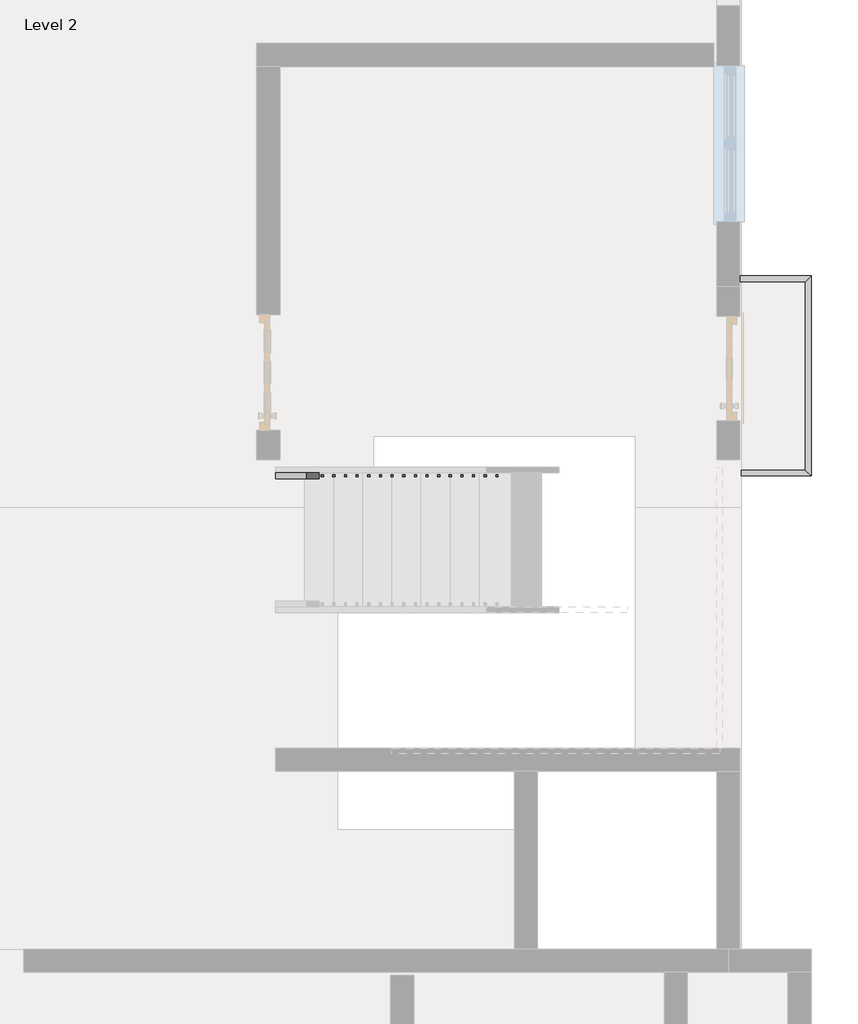
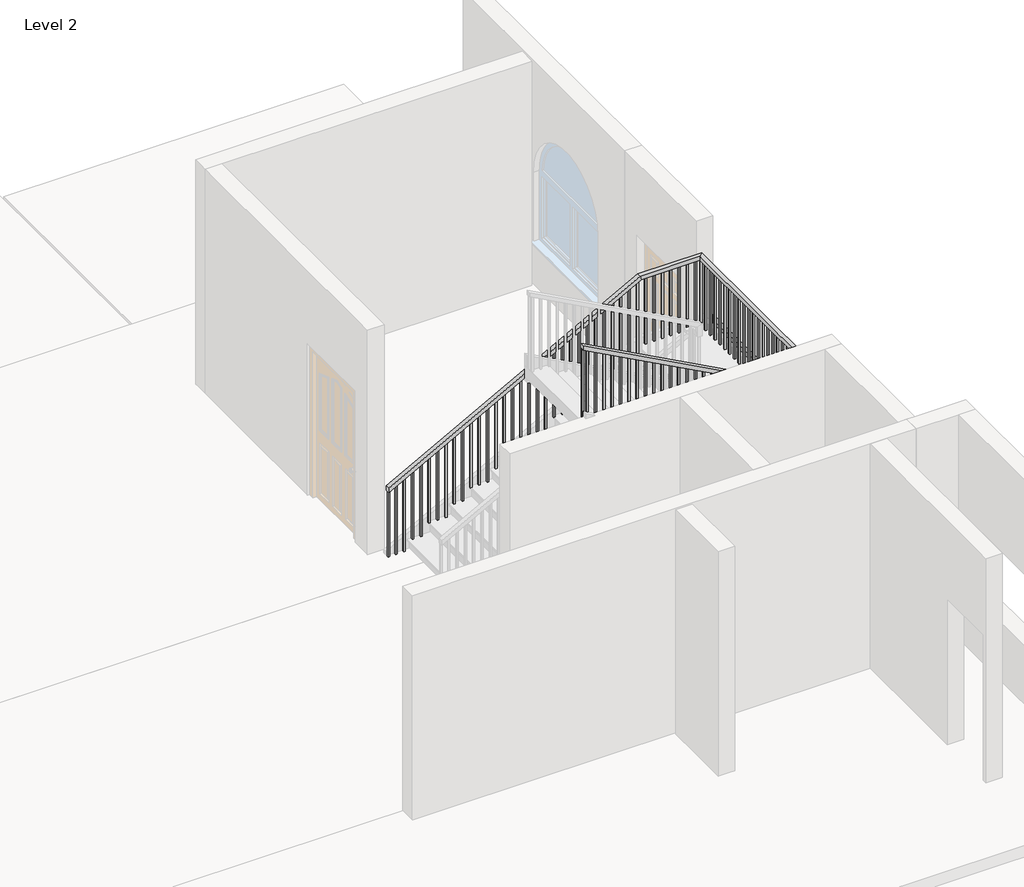
# One storey, part 6 of 7: 2 railings.
"""IFC4 building model written with IfcOpenShell, lengths in millimetres."""

from ifc_helpers import new_model, si_unit, frame, origin, place, context, project, spatial, polyline, outline, extrude, faceted_brep, element, save

model = new_model("IFC4")

# Units and contexts
model_context = context("Model", 3, world=origin())
ifc_project = project(units=[si_unit("LENGTHUNIT", "METRE", prefix="MILLI")], contexts=[model_context])

# Site, building, storey
site = spatial("IfcSite", under=ifc_project)
building = spatial("IfcBuilding", under=site)
storey = spatial("IfcBuildingStorey", under=building, Name="Level 2", Elevation=3048.0)

# Railings
placement = place(None, origin())
element("IfcRailing", 1, ObjectType="Handrail - Rectangular", at=placement, inside=storey, context=model_context, shape_type="SolidModel", body=[
    faceted_brep([(5863.1890963, 3183.81308, 3962.4), (5863.1890963, 3183.81308, 3911.6), (5863.1890963, 3133.01308, 3911.6), (5863.1890963, 3133.01308, 3962.4), (6485.4890963, 3183.81308, 3962.4), (6485.4890963, 3183.81308, 3911.6), (6434.6890963, 3133.01308, 3911.6), (6434.6890963, 3133.01308, 3962.4), (6485.4890963, 1439.3962251, 3962.4), (6485.4890963, 1439.3962251, 3911.6), (6434.6890963, 1490.1962251, 3911.6), (6434.6890963, 1490.1962251, 3962.4), (5875.8890963, 1439.3962251, 3962.4), (5875.8890963, 1490.1962251, 3962.4), (5875.8890963, 1490.1962251, 3911.6), (5875.8890963, 1439.3962251, 3911.6)], [[[0, 1, 2, 3]], [[1, 0, 4, 5]], [[2, 1, 5, 6]], [[3, 2, 6, 7]], [[0, 3, 7, 4]], [[5, 4, 8, 9]], [[6, 5, 9, 10]], [[7, 6, 10, 11]], [[4, 7, 11, 8]], [[12, 13, 14, 15]], [[9, 8, 12, 15]], [[10, 9, 15, 14]], [[11, 10, 14, 13]], [[8, 11, 13, 12]]]),
    extrude(outline(polyline([(5961.6140963, 1474.3212251), (5961.6140963, 1455.2712251), (5942.5640963, 1455.2712251), (5942.5640963, 1474.3212251), (5961.6140963, 1474.3212251)])), frame((0.0, 0.0, 3048.0), z_axis=(0.0, 0.0, 1.0), x_axis=(1.0, 0.0, 0.0)), (0.0, 0.0, 1.0), 863.6),
    extrude(outline(polyline([(6063.2140963, 1474.3212251), (6063.2140963, 1455.2712251), (6044.1640963, 1455.2712251), (6044.1640963, 1474.3212251), (6063.2140963, 1474.3212251)])), frame((0.0, 0.0, 3048.0), z_axis=(0.0, 0.0, 1.0), x_axis=(1.0, 0.0, 0.0)), (0.0, 0.0, 1.0), 863.6),
    extrude(outline(polyline([(6164.8140963, 1474.3212251), (6164.8140963, 1455.2712251), (6145.7640963, 1455.2712251), (6145.7640963, 1474.3212251), (6164.8140963, 1474.3212251)])), frame((0.0, 0.0, 3048.0), z_axis=(0.0, 0.0, 1.0), x_axis=(1.0, 0.0, 0.0)), (0.0, 0.0, 1.0), 863.6),
    extrude(outline(polyline([(6266.4140963, 1474.3212251), (6266.4140963, 1455.2712251), (6247.3640963, 1455.2712251), (6247.3640963, 1474.3212251), (6266.4140963, 1474.3212251)])), frame((0.0, 0.0, 3048.0), z_axis=(0.0, 0.0, 1.0), x_axis=(1.0, 0.0, 0.0)), (0.0, 0.0, 1.0), 863.6),
    extrude(outline(polyline([(6368.0140963, 1474.3212251), (6368.0140963, 1455.2712251), (6348.9640963, 1455.2712251), (6348.9640963, 1474.3212251), (6368.0140963, 1474.3212251)])), frame((0.0, 0.0, 3048.0), z_axis=(0.0, 0.0, 1.0), x_axis=(1.0, 0.0, 0.0)), (0.0, 0.0, 1.0), 863.6),
    extrude(outline(polyline([(6450.5640963, 1542.33808), (6469.6140963, 1542.33808), (6469.6140963, 1523.28808), (6450.5640963, 1523.28808), (6450.5640963, 1542.33808)])), frame((0.0, 0.0, 3048.0), z_axis=(0.0, 0.0, 1.0), x_axis=(1.0, 0.0, 0.0)), (0.0, 0.0, 1.0), 863.6),
    extrude(outline(polyline([(6450.5640963, 1643.93808), (6469.6140963, 1643.93808), (6469.6140963, 1624.88808), (6450.5640963, 1624.88808), (6450.5640963, 1643.93808)])), frame((0.0, 0.0, 3048.0), z_axis=(0.0, 0.0, 1.0), x_axis=(1.0, 0.0, 0.0)), (0.0, 0.0, 1.0), 863.6),
    extrude(outline(polyline([(6450.5640963, 1745.53808), (6469.6140963, 1745.53808), (6469.6140963, 1726.48808), (6450.5640963, 1726.48808), (6450.5640963, 1745.53808)])), frame((0.0, 0.0, 3048.0), z_axis=(0.0, 0.0, 1.0), x_axis=(1.0, 0.0, 0.0)), (0.0, 0.0, 1.0), 863.6),
    extrude(outline(polyline([(6450.5640963, 1847.13808), (6469.6140963, 1847.13808), (6469.6140963, 1828.08808), (6450.5640963, 1828.08808), (6450.5640963, 1847.13808)])), frame((0.0, 0.0, 3048.0), z_axis=(0.0, 0.0, 1.0), x_axis=(1.0, 0.0, 0.0)), (0.0, 0.0, 1.0), 863.6),
    extrude(outline(polyline([(6450.5640963, 1948.73808), (6469.6140963, 1948.73808), (6469.6140963, 1929.68808), (6450.5640963, 1929.68808), (6450.5640963, 1948.73808)])), frame((0.0, 0.0, 3048.0), z_axis=(0.0, 0.0, 1.0), x_axis=(1.0, 0.0, 0.0)), (0.0, 0.0, 1.0), 863.6),
    extrude(outline(polyline([(6450.5640963, 2050.33808), (6469.6140963, 2050.33808), (6469.6140963, 2031.28808), (6450.5640963, 2031.28808), (6450.5640963, 2050.33808)])), frame((0.0, 0.0, 3048.0), z_axis=(0.0, 0.0, 1.0), x_axis=(1.0, 0.0, 0.0)), (0.0, 0.0, 1.0), 863.6),
    extrude(outline(polyline([(6450.5640963, 2151.93808), (6469.6140963, 2151.93808), (6469.6140963, 2132.88808), (6450.5640963, 2132.88808), (6450.5640963, 2151.93808)])), frame((0.0, 0.0, 3048.0), z_axis=(0.0, 0.0, 1.0), x_axis=(1.0, 0.0, 0.0)), (0.0, 0.0, 1.0), 863.6),
    extrude(outline(polyline([(6450.5640963, 2253.53808), (6469.6140963, 2253.53808), (6469.6140963, 2234.48808), (6450.5640963, 2234.48808), (6450.5640963, 2253.53808)])), frame((0.0, 0.0, 3048.0), z_axis=(0.0, 0.0, 1.0), x_axis=(1.0, 0.0, 0.0)), (0.0, 0.0, 1.0), 863.6),
    extrude(outline(polyline([(6450.5640963, 2355.13808), (6469.6140963, 2355.13808), (6469.6140963, 2336.08808), (6450.5640963, 2336.08808), (6450.5640963, 2355.13808)])), frame((0.0, 0.0, 3048.0), z_axis=(0.0, 0.0, 1.0), x_axis=(1.0, 0.0, 0.0)), (0.0, 0.0, 1.0), 863.6),
    extrude(outline(polyline([(6450.5640963, 2456.73808), (6469.6140963, 2456.73808), (6469.6140963, 2437.68808), (6450.5640963, 2437.68808), (6450.5640963, 2456.73808)])), frame((0.0, 0.0, 3048.0), z_axis=(0.0, 0.0, 1.0), x_axis=(1.0, 0.0, 0.0)), (0.0, 0.0, 1.0), 863.6),
    extrude(outline(polyline([(6450.5640963, 2558.33808), (6469.6140963, 2558.33808), (6469.6140963, 2539.28808), (6450.5640963, 2539.28808), (6450.5640963, 2558.33808)])), frame((0.0, 0.0, 3048.0), z_axis=(0.0, 0.0, 1.0), x_axis=(1.0, 0.0, 0.0)), (0.0, 0.0, 1.0), 863.6),
    extrude(outline(polyline([(6450.5640963, 2659.93808), (6469.6140963, 2659.93808), (6469.6140963, 2640.88808), (6450.5640963, 2640.88808), (6450.5640963, 2659.93808)])), frame((0.0, 0.0, 3048.0), z_axis=(0.0, 0.0, 1.0), x_axis=(1.0, 0.0, 0.0)), (0.0, 0.0, 1.0), 863.6),
    extrude(outline(polyline([(6450.5640963, 2761.53808), (6469.6140963, 2761.53808), (6469.6140963, 2742.48808), (6450.5640963, 2742.48808), (6450.5640963, 2761.53808)])), frame((0.0, 0.0, 3048.0), z_axis=(0.0, 0.0, 1.0), x_axis=(1.0, 0.0, 0.0)), (0.0, 0.0, 1.0), 863.6),
    extrude(outline(polyline([(6450.5640963, 2863.13808), (6469.6140963, 2863.13808), (6469.6140963, 2844.08808), (6450.5640963, 2844.08808), (6450.5640963, 2863.13808)])), frame((0.0, 0.0, 3048.0), z_axis=(0.0, 0.0, 1.0), x_axis=(1.0, 0.0, 0.0)), (0.0, 0.0, 1.0), 863.6),
    extrude(outline(polyline([(6450.5640963, 2964.73808), (6469.6140963, 2964.73808), (6469.6140963, 2945.68808), (6450.5640963, 2945.68808), (6450.5640963, 2964.73808)])), frame((0.0, 0.0, 3048.0), z_axis=(0.0, 0.0, 1.0), x_axis=(1.0, 0.0, 0.0)), (0.0, 0.0, 1.0), 863.6),
    extrude(outline(polyline([(6450.5640963, 3066.33808), (6469.6140963, 3066.33808), (6469.6140963, 3047.28808), (6450.5640963, 3047.28808), (6450.5640963, 3066.33808)])), frame((0.0, 0.0, 3048.0), z_axis=(0.0, 0.0, 1.0), x_axis=(1.0, 0.0, 0.0)), (0.0, 0.0, 1.0), 863.6),
    extrude(outline(polyline([(6361.6640963, 3148.88808), (6361.6640963, 3167.93808), (6380.7140963, 3167.93808), (6380.7140963, 3148.88808), (6361.6640963, 3148.88808)])), frame((0.0, 0.0, 3048.0), z_axis=(0.0, 0.0, 1.0), x_axis=(1.0, 0.0, 0.0)), (0.0, 0.0, 1.0), 863.6),
    extrude(outline(polyline([(6260.0640963, 3148.88808), (6260.0640963, 3167.93808), (6279.1140963, 3167.93808), (6279.1140963, 3148.88808), (6260.0640963, 3148.88808)])), frame((0.0, 0.0, 3048.0), z_axis=(0.0, 0.0, 1.0), x_axis=(1.0, 0.0, 0.0)), (0.0, 0.0, 1.0), 863.6),
    extrude(outline(polyline([(6158.4640963, 3148.88808), (6158.4640963, 3167.93808), (6177.5140963, 3167.93808), (6177.5140963, 3148.88808), (6158.4640963, 3148.88808)])), frame((0.0, 0.0, 3048.0), z_axis=(0.0, 0.0, 1.0), x_axis=(1.0, 0.0, 0.0)), (0.0, 0.0, 1.0), 863.6),
    extrude(outline(polyline([(6056.8640963, 3148.88808), (6056.8640963, 3167.93808), (6075.9140963, 3167.93808), (6075.9140963, 3148.88808), (6056.8640963, 3148.88808)])), frame((0.0, 0.0, 3048.0), z_axis=(0.0, 0.0, 1.0), x_axis=(1.0, 0.0, 0.0)), (0.0, 0.0, 1.0), 863.6),
    extrude(outline(polyline([(5955.2640963, 3148.88808), (5955.2640963, 3167.93808), (5974.3140963, 3167.93808), (5974.3140963, 3148.88808), (5955.2640963, 3148.88808)])), frame((0.0, 0.0, 3048.0), z_axis=(0.0, 0.0, 1.0), x_axis=(1.0, 0.0, 0.0)), (0.0, 0.0, 1.0), 863.6),
    extrude(outline(polyline([(6450.5640963, 1474.3212251), (6469.6140963, 1474.3212251), (6469.6140963, 1455.2712251), (6450.5640963, 1455.2712251), (6450.5640963, 1474.3212251)])), frame((0.0, 0.0, 3048.0), z_axis=(0.0, 0.0, 1.0), x_axis=(1.0, 0.0, 0.0)), (0.0, 0.0, 1.0), 863.6),
    extrude(outline(polyline([(6450.5640963, 3148.88808), (6450.5640963, 3167.93808), (6469.6140963, 3167.93808), (6469.6140963, 3148.88808), (6450.5640963, 3148.88808)])), frame((0.0, 0.0, 3048.0), z_axis=(0.0, 0.0, 1.0), x_axis=(1.0, 0.0, 0.0)), (0.0, 0.0, 1.0), 863.6),
    extrude(outline(polyline([(5894.9390963, 1474.3212251), (5894.9390963, 1455.2712251), (5875.8890963, 1455.2712251), (5875.8890963, 1474.3212251), (5894.9390963, 1474.3212251)])), frame((0.0, 0.0, 3048.0), z_axis=(0.0, 0.0, 1.0), x_axis=(1.0, 0.0, 0.0)), (0.0, 0.0, 1.0), 863.6),
    extrude(outline(polyline([(5863.1890963, 3148.88808), (5863.1890963, 3167.93808), (5882.2390963, 3167.93808), (5882.2390963, 3148.88808), (5863.1890963, 3148.88808)])), frame((0.0, 0.0, 3048.0), z_axis=(0.0, 0.0, 1.0), x_axis=(1.0, 0.0, 0.0)), (0.0, 0.0, 1.0), 863.6),
])
element("IfcRailing", 2, ObjectType="Handrail - Rectangular", at=placement, inside=storey, context=model_context, shape_type="SolidModel", body=[
    faceted_brep([(1811.8890963, 1464.7962251, 4100.9454545), (1811.8890963, 1464.7962251, 4043.1709673), (1811.8890963, 1413.9962251, 4043.1709673), (1811.8890963, 1413.9962251, 4100.9454545), (4881.0326586, 1464.7962251, 5763.4909091), (4893.9079172, 1464.7962251, 5712.6909091), (4893.9079172, 1413.9962251, 5712.6909091), (4881.0326586, 1413.9962251, 5763.4909091), (5659.9890963, 1464.7962251, 5763.4909091), (5659.9890963, 1464.7962251, 5712.6909091), (5609.1890963, 1413.9962251, 5712.6909091), (5609.1890963, 1413.9962251, 5763.4909091), (5659.9890963, -935.5037749, 5763.4909091), (5659.9890963, -935.5037749, 5712.6909091), (5609.1890963, -884.7037749, 5712.6909091), (5609.1890963, -884.7037749, 5763.4909091), (5137.6756039, -935.5037749, 5763.4909091), (5124.8392301, -935.5037749, 5712.6909091), (5124.8392301, -884.7037749, 5712.6909091), (5137.6756039, -884.7037749, 5763.4909091), (2827.8890963, -935.5037749, 7010.4), (2827.8890963, -884.7037749, 7010.4), (2827.8890963, -884.7037749, 6952.6704456), (2827.8890963, -935.5037749, 6952.6704456)], [[[0, 1, 2, 3]], [[1, 0, 4, 5]], [[2, 1, 5, 6]], [[3, 2, 6, 7]], [[0, 3, 7, 4]], [[5, 4, 8, 9]], [[6, 5, 9, 10]], [[7, 6, 10, 11]], [[4, 7, 11, 8]], [[9, 8, 12, 13]], [[10, 9, 13, 14]], [[11, 10, 14, 15]], [[8, 11, 15, 12]], [[13, 12, 16, 17]], [[14, 13, 17, 18]], [[15, 14, 18, 19]], [[12, 15, 19, 16]], [[20, 21, 22, 23]], [[17, 16, 20, 23]], [[18, 17, 23, 22]], [[19, 18, 22, 21]], [[16, 19, 21, 20]]]),
    extrude(outline(polyline([(6923.5858236, 2881.8640963), (5957.4545455, 2881.8640963), (5957.4545455, 2900.9140963), (6913.2664983, 2900.9140963), (6923.5858236, 2881.8640963)])), frame((0.0, -919.6287749, 0.0), z_axis=(0.0, 1.0, 0.0), x_axis=(0.0, 0.0, 1.0)), (0.0, 0.0, 1.0), 19.05),
    extrude(outline(polyline([(6868.5494219, 2983.4640963), (5957.4545455, 2983.4640963), (5957.4545455, 3002.5140963), (6858.2300965, 3002.5140963), (6868.5494219, 2983.4640963)])), frame((0.0, -919.6287749, 0.0), z_axis=(0.0, 1.0, 0.0), x_axis=(0.0, 0.0, 1.0)), (0.0, 0.0, 1.0), 19.05),
    extrude(outline(polyline([(6813.8377681, 3085.0640963), (5818.9090909, 3085.0640963), (5818.9090909, 3104.1140963), (6803.553866, 3104.1140963), (6813.8377681, 3085.0640963)])), frame((0.0, -919.6287749, 0.0), z_axis=(0.0, 1.0, 0.0), x_axis=(0.0, 0.0, 1.0)), (0.0, 0.0, 1.0), 19.05),
    extrude(outline(polyline([(6758.9902905, 3186.6640963), (5818.9090909, 3186.6640963), (5818.9090909, 3205.7140963), (6748.7063885, 3205.7140963), (6758.9902905, 3186.6640963)])), frame((0.0, -919.6287749, 0.0), z_axis=(0.0, 1.0, 0.0), x_axis=(0.0, 0.0, 1.0)), (0.0, 0.0, 1.0), 19.05),
    extrude(outline(polyline([(6704.1428129, 3288.2640963), (5818.9090909, 3288.2640963), (5818.9090909, 3307.3140963), (6693.8589109, 3307.3140963), (6704.1428129, 3288.2640963)])), frame((0.0, -919.6287749, 0.0), z_axis=(0.0, 1.0, 0.0), x_axis=(0.0, 0.0, 1.0)), (0.0, 0.0, 1.0), 19.05),
    extrude(outline(polyline([(6649.2953354, 3389.8640963), (5680.3636364, 3389.8640963), (5680.3636364, 3408.9140963), (6639.0114333, 3408.9140963), (6649.2953354, 3389.8640963)])), frame((0.0, -919.6287749, 0.0), z_axis=(0.0, 1.0, 0.0), x_axis=(0.0, 0.0, 1.0)), (0.0, 0.0, 1.0), 19.05),
    extrude(outline(polyline([(6594.4478578, 3491.4640963), (5680.3636364, 3491.4640963), (5680.3636364, 3510.5140963), (6584.1639558, 3510.5140963), (6594.4478578, 3491.4640963)])), frame((0.0, -919.6287749, 0.0), z_axis=(0.0, 1.0, 0.0), x_axis=(0.0, 0.0, 1.0)), (0.0, 0.0, 1.0), 19.05),
    extrude(outline(polyline([(6539.6003803, 3593.0640963), (5541.8181818, 3593.0640963), (5541.8181818, 3612.1140963), (6529.3164782, 3612.1140963), (6539.6003803, 3593.0640963)])), frame((0.0, -919.6287749, 0.0), z_axis=(0.0, 1.0, 0.0), x_axis=(0.0, 0.0, 1.0)), (0.0, 0.0, 1.0), 19.05),
    extrude(outline(polyline([(6484.7529027, 3694.6640963), (5541.8181818, 3694.6640963), (5541.8181818, 3713.7140963), (6474.4690007, 3713.7140963), (6484.7529027, 3694.6640963)])), frame((0.0, -919.6287749, 0.0), z_axis=(0.0, 1.0, 0.0), x_axis=(0.0, 0.0, 1.0)), (0.0, 0.0, 1.0), 19.05),
    extrude(outline(polyline([(6429.9054252, 3796.2640963), (5541.8181818, 3796.2640963), (5541.8181818, 3815.3140963), (6419.6215231, 3815.3140963), (6429.9054252, 3796.2640963)])), frame((0.0, -919.6287749, 0.0), z_axis=(0.0, 1.0, 0.0), x_axis=(0.0, 0.0, 1.0)), (0.0, 0.0, 1.0), 19.05),
    extrude(outline(polyline([(6375.1307062, 3897.8640963), (5403.2727273, 3897.8640963), (5403.2727273, 3916.9140963), (6364.8113809, 3916.9140963), (6375.1307062, 3897.8640963)])), frame((0.0, -919.6287749, 0.0), z_axis=(0.0, 1.0, 0.0), x_axis=(0.0, 0.0, 1.0)), (0.0, 0.0, 1.0), 19.05),
    extrude(outline(polyline([(6320.0943044, 3999.4640963), (5403.2727273, 3999.4640963), (5403.2727273, 4018.5140963), (6309.7749791, 4018.5140963), (6320.0943044, 3999.4640963)])), frame((0.0, -919.6287749, 0.0), z_axis=(0.0, 1.0, 0.0), x_axis=(0.0, 0.0, 1.0)), (0.0, 0.0, 1.0), 19.05),
    extrude(outline(polyline([(6265.3629925, 4101.0640963), (5264.7272727, 4101.0640963), (5264.7272727, 4120.1140963), (6255.0790904, 4120.1140963), (6265.3629925, 4101.0640963)])), frame((0.0, -919.6287749, 0.0), z_axis=(0.0, 1.0, 0.0), x_axis=(0.0, 0.0, 1.0)), (0.0, 0.0, 1.0), 19.05),
    extrude(outline(polyline([(6210.5155149, 4202.6640963), (5264.7272727, 4202.6640963), (5264.7272727, 4221.7140963), (6200.2316129, 4221.7140963), (6210.5155149, 4202.6640963)])), frame((0.0, -919.6287749, 0.0), z_axis=(0.0, 1.0, 0.0), x_axis=(0.0, 0.0, 1.0)), (0.0, 0.0, 1.0), 19.05),
    extrude(outline(polyline([(6155.6680374, 4304.2640963), (5264.7272727, 4304.2640963), (5264.7272727, 4323.3140963), (6145.3841353, 4323.3140963), (6155.6680374, 4304.2640963)])), frame((0.0, -919.6287749, 0.0), z_axis=(0.0, 1.0, 0.0), x_axis=(0.0, 0.0, 1.0)), (0.0, 0.0, 1.0), 19.05),
    extrude(outline(polyline([(6100.8205598, 4405.8640963), (5126.1818182, 4405.8640963), (5126.1818182, 4424.9140963), (6090.5366578, 4424.9140963), (6100.8205598, 4405.8640963)])), frame((0.0, -919.6287749, 0.0), z_axis=(0.0, 1.0, 0.0), x_axis=(0.0, 0.0, 1.0)), (0.0, 0.0, 1.0), 19.05),
    extrude(outline(polyline([(6045.9730823, 4507.4640963), (5126.1818182, 4507.4640963), (5126.1818182, 4526.5140963), (6035.6891802, 4526.5140963), (6045.9730823, 4507.4640963)])), frame((0.0, -919.6287749, 0.0), z_axis=(0.0, 1.0, 0.0), x_axis=(0.0, 0.0, 1.0)), (0.0, 0.0, 1.0), 19.05),
    extrude(outline(polyline([(5991.1256047, 4609.0640963), (4987.6363636, 4609.0640963), (4987.6363636, 4628.1140963), (5980.8417027, 4628.1140963), (5991.1256047, 4609.0640963)])), frame((0.0, -919.6287749, 0.0), z_axis=(0.0, 1.0, 0.0), x_axis=(0.0, 0.0, 1.0)), (0.0, 0.0, 1.0), 19.05),
    extrude(outline(polyline([(5936.2781272, 4710.6640963), (4987.6363636, 4710.6640963), (4987.6363636, 4729.7140963), (5925.9942251, 4729.7140963), (5936.2781272, 4710.6640963)])), frame((0.0, -919.6287749, 0.0), z_axis=(0.0, 1.0, 0.0), x_axis=(0.0, 0.0, 1.0)), (0.0, 0.0, 1.0), 19.05),
    extrude(outline(polyline([(5881.4306496, 4812.2640963), (4987.6363636, 4812.2640963), (4987.6363636, 4831.3140963), (5871.1467476, 4831.3140963), (5881.4306496, 4812.2640963)])), frame((0.0, -919.6287749, 0.0), z_axis=(0.0, 1.0, 0.0), x_axis=(0.0, 0.0, 1.0)), (0.0, 0.0, 1.0), 19.05),
    extrude(outline(polyline([(5826.583172, 4913.8640963), (4849.0909091, 4913.8640963), (4849.0909091, 4932.9140963), (5816.29927, 4932.9140963), (5826.583172, 4913.8640963)])), frame((0.0, -919.6287749, 0.0), z_axis=(0.0, 1.0, 0.0), x_axis=(0.0, 0.0, 1.0)), (0.0, 0.0, 1.0), 19.05),
    extrude(outline(polyline([(5771.7356945, 5015.4640963), (4849.0909091, 5015.4640963), (4849.0909091, 5034.5140963), (5761.4517924, 5034.5140963), (5771.7356945, 5015.4640963)])), frame((0.0, -919.6287749, 0.0), z_axis=(0.0, 1.0, 0.0), x_axis=(0.0, 0.0, 1.0)), (0.0, 0.0, 1.0), 19.05),
    extrude(outline(polyline([(5716.8882169, 5117.0640963), (4849.0909091, 5117.0640963), (4849.0909091, 5136.1140963), (5706.6043149, 5136.1140963), (5716.8882169, 5117.0640963)])), frame((0.0, -919.6287749, 0.0), z_axis=(0.0, 1.0, 0.0), x_axis=(0.0, 0.0, 1.0)), (0.0, 0.0, 1.0), 19.05),
    extrude(outline(polyline([(5237.7140963, -919.6287749), (5218.6640963, -919.6287749), (5218.6640963, -900.5787749), (5237.7140963, -900.5787749), (5237.7140963, -919.6287749)])), frame((0.0, 0.0, 4849.0909091), z_axis=(0.0, 0.0, 1.0), x_axis=(1.0, 0.0, 0.0)), (0.0, 0.0, 1.0), 863.6),
    extrude(outline(polyline([(5339.3140963, -919.6287749), (5320.2640963, -919.6287749), (5320.2640963, -900.5787749), (5339.3140963, -900.5787749), (5339.3140963, -919.6287749)])), frame((0.0, 0.0, 4849.0909091), z_axis=(0.0, 0.0, 1.0), x_axis=(1.0, 0.0, 0.0)), (0.0, 0.0, 1.0), 863.6),
    extrude(outline(polyline([(5440.9140963, -919.6287749), (5421.8640963, -919.6287749), (5421.8640963, -900.5787749), (5440.9140963, -900.5787749), (5440.9140963, -919.6287749)])), frame((0.0, 0.0, 4849.0909091), z_axis=(0.0, 0.0, 1.0), x_axis=(1.0, 0.0, 0.0)), (0.0, 0.0, 1.0), 863.6),
    extrude(outline(polyline([(5542.5140963, -919.6287749), (5523.4640963, -919.6287749), (5523.4640963, -900.5787749), (5542.5140963, -900.5787749), (5542.5140963, -919.6287749)])), frame((0.0, 0.0, 4849.0909091), z_axis=(0.0, 0.0, 1.0), x_axis=(1.0, 0.0, 0.0)), (0.0, 0.0, 1.0), 863.6),
    extrude(outline(polyline([(5644.1140963, -887.8787749), (5644.1140963, -906.9287749), (5625.0640963, -906.9287749), (5625.0640963, -887.8787749), (5644.1140963, -887.8787749)])), frame((0.0, 0.0, 4849.0909091), z_axis=(0.0, 0.0, 1.0), x_axis=(1.0, 0.0, 0.0)), (0.0, 0.0, 1.0), 863.6),
    extrude(outline(polyline([(5644.1140963, -786.2787749), (5644.1140963, -805.3287749), (5625.0640963, -805.3287749), (5625.0640963, -786.2787749), (5644.1140963, -786.2787749)])), frame((0.0, 0.0, 4849.0909091), z_axis=(0.0, 0.0, 1.0), x_axis=(1.0, 0.0, 0.0)), (0.0, 0.0, 1.0), 863.6),
    extrude(outline(polyline([(5644.1140963, -684.6787749), (5644.1140963, -703.7287749), (5625.0640963, -703.7287749), (5625.0640963, -684.6787749), (5644.1140963, -684.6787749)])), frame((0.0, 0.0, 4849.0909091), z_axis=(0.0, 0.0, 1.0), x_axis=(1.0, 0.0, 0.0)), (0.0, 0.0, 1.0), 863.6),
    extrude(outline(polyline([(5644.1140963, -583.0787749), (5644.1140963, -602.1287749), (5625.0640963, -602.1287749), (5625.0640963, -583.0787749), (5644.1140963, -583.0787749)])), frame((0.0, 0.0, 4849.0909091), z_axis=(0.0, 0.0, 1.0), x_axis=(1.0, 0.0, 0.0)), (0.0, 0.0, 1.0), 863.6),
    extrude(outline(polyline([(5644.1140963, -481.4787749), (5644.1140963, -500.5287749), (5625.0640963, -500.5287749), (5625.0640963, -481.4787749), (5644.1140963, -481.4787749)])), frame((0.0, 0.0, 4849.0909091), z_axis=(0.0, 0.0, 1.0), x_axis=(1.0, 0.0, 0.0)), (0.0, 0.0, 1.0), 863.6),
    extrude(outline(polyline([(5644.1140963, -379.8787749), (5644.1140963, -398.9287749), (5625.0640963, -398.9287749), (5625.0640963, -379.8787749), (5644.1140963, -379.8787749)])), frame((0.0, 0.0, 4849.0909091), z_axis=(0.0, 0.0, 1.0), x_axis=(1.0, 0.0, 0.0)), (0.0, 0.0, 1.0), 863.6),
    extrude(outline(polyline([(5644.1140963, -278.2787749), (5644.1140963, -297.3287749), (5625.0640963, -297.3287749), (5625.0640963, -278.2787749), (5644.1140963, -278.2787749)])), frame((0.0, 0.0, 4849.0909091), z_axis=(0.0, 0.0, 1.0), x_axis=(1.0, 0.0, 0.0)), (0.0, 0.0, 1.0), 863.6),
    extrude(outline(polyline([(5644.1140963, -176.6787749), (5644.1140963, -195.7287749), (5625.0640963, -195.7287749), (5625.0640963, -176.6787749), (5644.1140963, -176.6787749)])), frame((0.0, 0.0, 4849.0909091), z_axis=(0.0, 0.0, 1.0), x_axis=(1.0, 0.0, 0.0)), (0.0, 0.0, 1.0), 863.6),
    extrude(outline(polyline([(5644.1140963, -75.0787749), (5644.1140963, -94.1287749), (5625.0640963, -94.1287749), (5625.0640963, -75.0787749), (5644.1140963, -75.0787749)])), frame((0.0, 0.0, 4849.0909091), z_axis=(0.0, 0.0, 1.0), x_axis=(1.0, 0.0, 0.0)), (0.0, 0.0, 1.0), 863.6),
    extrude(outline(polyline([(5644.1140963, 26.5212251), (5644.1140963, 7.4712251), (5625.0640963, 7.4712251), (5625.0640963, 26.5212251), (5644.1140963, 26.5212251)])), frame((0.0, 0.0, 4849.0909091), z_axis=(0.0, 0.0, 1.0), x_axis=(1.0, 0.0, 0.0)), (0.0, 0.0, 1.0), 863.6),
    extrude(outline(polyline([(5644.1140963, 128.1212251), (5644.1140963, 109.0712251), (5625.0640963, 109.0712251), (5625.0640963, 128.1212251), (5644.1140963, 128.1212251)])), frame((0.0, 0.0, 4849.0909091), z_axis=(0.0, 0.0, 1.0), x_axis=(1.0, 0.0, 0.0)), (0.0, 0.0, 1.0), 863.6),
    extrude(outline(polyline([(5644.1140963, 229.7212251), (5644.1140963, 210.6712251), (5625.0640963, 210.6712251), (5625.0640963, 229.7212251), (5644.1140963, 229.7212251)])), frame((0.0, 0.0, 4849.0909091), z_axis=(0.0, 0.0, 1.0), x_axis=(1.0, 0.0, 0.0)), (0.0, 0.0, 1.0), 863.6),
    extrude(outline(polyline([(5644.1140963, 331.3212251), (5644.1140963, 312.2712251), (5625.0640963, 312.2712251), (5625.0640963, 331.3212251), (5644.1140963, 331.3212251)])), frame((0.0, 0.0, 4849.0909091), z_axis=(0.0, 0.0, 1.0), x_axis=(1.0, 0.0, 0.0)), (0.0, 0.0, 1.0), 863.6),
    extrude(outline(polyline([(5644.1140963, 432.9212251), (5644.1140963, 413.8712251), (5625.0640963, 413.8712251), (5625.0640963, 432.9212251), (5644.1140963, 432.9212251)])), frame((0.0, 0.0, 4849.0909091), z_axis=(0.0, 0.0, 1.0), x_axis=(1.0, 0.0, 0.0)), (0.0, 0.0, 1.0), 863.6),
    extrude(outline(polyline([(5644.1140963, 534.5212251), (5644.1140963, 515.4712251), (5625.0640963, 515.4712251), (5625.0640963, 534.5212251), (5644.1140963, 534.5212251)])), frame((0.0, 0.0, 4849.0909091), z_axis=(0.0, 0.0, 1.0), x_axis=(1.0, 0.0, 0.0)), (0.0, 0.0, 1.0), 863.6),
    extrude(outline(polyline([(5644.1140963, 636.1212251), (5644.1140963, 617.0712251), (5625.0640963, 617.0712251), (5625.0640963, 636.1212251), (5644.1140963, 636.1212251)])), frame((0.0, 0.0, 4849.0909091), z_axis=(0.0, 0.0, 1.0), x_axis=(1.0, 0.0, 0.0)), (0.0, 0.0, 1.0), 863.6),
    extrude(outline(polyline([(5644.1140963, 737.7212251), (5644.1140963, 718.6712251), (5625.0640963, 718.6712251), (5625.0640963, 737.7212251), (5644.1140963, 737.7212251)])), frame((0.0, 0.0, 4849.0909091), z_axis=(0.0, 0.0, 1.0), x_axis=(1.0, 0.0, 0.0)), (0.0, 0.0, 1.0), 863.6),
    extrude(outline(polyline([(5644.1140963, 839.3212251), (5644.1140963, 820.2712251), (5625.0640963, 820.2712251), (5625.0640963, 839.3212251), (5644.1140963, 839.3212251)])), frame((0.0, 0.0, 4849.0909091), z_axis=(0.0, 0.0, 1.0), x_axis=(1.0, 0.0, 0.0)), (0.0, 0.0, 1.0), 863.6),
    extrude(outline(polyline([(5644.1140963, 940.9212251), (5644.1140963, 921.8712251), (5625.0640963, 921.8712251), (5625.0640963, 940.9212251), (5644.1140963, 940.9212251)])), frame((0.0, 0.0, 4849.0909091), z_axis=(0.0, 0.0, 1.0), x_axis=(1.0, 0.0, 0.0)), (0.0, 0.0, 1.0), 863.6),
    extrude(outline(polyline([(5644.1140963, 1042.5212251), (5644.1140963, 1023.4712251), (5625.0640963, 1023.4712251), (5625.0640963, 1042.5212251), (5644.1140963, 1042.5212251)])), frame((0.0, 0.0, 4849.0909091), z_axis=(0.0, 0.0, 1.0), x_axis=(1.0, 0.0, 0.0)), (0.0, 0.0, 1.0), 863.6),
    extrude(outline(polyline([(5644.1140963, 1144.1212251), (5644.1140963, 1125.0712251), (5625.0640963, 1125.0712251), (5625.0640963, 1144.1212251), (5644.1140963, 1144.1212251)])), frame((0.0, 0.0, 4849.0909091), z_axis=(0.0, 0.0, 1.0), x_axis=(1.0, 0.0, 0.0)), (0.0, 0.0, 1.0), 863.6),
    extrude(outline(polyline([(5644.1140963, 1245.7212251), (5644.1140963, 1226.6712251), (5625.0640963, 1226.6712251), (5625.0640963, 1245.7212251), (5644.1140963, 1245.7212251)])), frame((0.0, 0.0, 4849.0909091), z_axis=(0.0, 0.0, 1.0), x_axis=(1.0, 0.0, 0.0)), (0.0, 0.0, 1.0), 863.6),
    extrude(outline(polyline([(5644.1140963, 1347.3212251), (5644.1140963, 1328.2712251), (5625.0640963, 1328.2712251), (5625.0640963, 1347.3212251), (5644.1140963, 1347.3212251)])), frame((0.0, 0.0, 4849.0909091), z_axis=(0.0, 0.0, 1.0), x_axis=(1.0, 0.0, 0.0)), (0.0, 0.0, 1.0), 863.6),
    extrude(outline(polyline([(5561.5640963, 1448.9212251), (5580.6140963, 1448.9212251), (5580.6140963, 1429.8712251), (5561.5640963, 1429.8712251), (5561.5640963, 1448.9212251)])), frame((0.0, 0.0, 4849.0909091), z_axis=(0.0, 0.0, 1.0), x_axis=(1.0, 0.0, 0.0)), (0.0, 0.0, 1.0), 863.6),
    extrude(outline(polyline([(5459.9640963, 1448.9212251), (5479.0140963, 1448.9212251), (5479.0140963, 1429.8712251), (5459.9640963, 1429.8712251), (5459.9640963, 1448.9212251)])), frame((0.0, 0.0, 4849.0909091), z_axis=(0.0, 0.0, 1.0), x_axis=(1.0, 0.0, 0.0)), (0.0, 0.0, 1.0), 863.6),
    extrude(outline(polyline([(5358.3640963, 1448.9212251), (5377.4140963, 1448.9212251), (5377.4140963, 1429.8712251), (5358.3640963, 1429.8712251), (5358.3640963, 1448.9212251)])), frame((0.0, 0.0, 4849.0909091), z_axis=(0.0, 0.0, 1.0), x_axis=(1.0, 0.0, 0.0)), (0.0, 0.0, 1.0), 863.6),
    extrude(outline(polyline([(5256.7640963, 1448.9212251), (5275.8140963, 1448.9212251), (5275.8140963, 1429.8712251), (5256.7640963, 1429.8712251), (5256.7640963, 1448.9212251)])), frame((0.0, 0.0, 4849.0909091), z_axis=(0.0, 0.0, 1.0), x_axis=(1.0, 0.0, 0.0)), (0.0, 0.0, 1.0), 863.6),
    extrude(outline(polyline([(5155.1640963, 1448.9212251), (5174.2140963, 1448.9212251), (5174.2140963, 1429.8712251), (5155.1640963, 1429.8712251), (5155.1640963, 1448.9212251)])), frame((0.0, 0.0, 4849.0909091), z_axis=(0.0, 0.0, 1.0), x_axis=(1.0, 0.0, 0.0)), (0.0, 0.0, 1.0), 863.6),
    extrude(outline(polyline([(5053.5640963, 1448.9212251), (5072.6140963, 1448.9212251), (5072.6140963, 1429.8712251), (5053.5640963, 1429.8712251), (5053.5640963, 1448.9212251)])), frame((0.0, 0.0, 4849.0909091), z_axis=(0.0, 0.0, 1.0), x_axis=(1.0, 0.0, 0.0)), (0.0, 0.0, 1.0), 863.6),
    extrude(outline(polyline([(4951.9640963, 1448.9212251), (4971.0140963, 1448.9212251), (4971.0140963, 1429.8712251), (4951.9640963, 1429.8712251), (4951.9640963, 1448.9212251)])), frame((0.0, 0.0, 4849.0909091), z_axis=(0.0, 0.0, 1.0), x_axis=(1.0, 0.0, 0.0)), (0.0, 0.0, 1.0), 863.6),
    extrude(outline(polyline([(5689.1033577, 4850.3640963), (4710.5454545, 4850.3640963), (4710.5454545, 4869.4140963), (5699.422683, 4869.4140963), (5689.1033577, 4850.3640963)])), frame((0.0, 1429.8712251, 0.0), z_axis=(0.0, 1.0, 0.0), x_axis=(0.0, 0.0, 1.0)), (0.0, 0.0, 1.0), 19.05),
    extrude(outline(polyline([(5634.0669559, 4748.7640963), (4710.5454545, 4748.7640963), (4710.5454545, 4767.8140963), (5644.3862812, 4767.8140963), (5634.0669559, 4748.7640963)])), frame((0.0, 1429.8712251, 0.0), z_axis=(0.0, 1.0, 0.0), x_axis=(0.0, 0.0, 1.0)), (0.0, 0.0, 1.0), 19.05),
    extrude(outline(polyline([(5579.0305541, 4647.1640963), (4710.5454545, 4647.1640963), (4710.5454545, 4666.2140963), (5589.3498795, 4666.2140963), (5579.0305541, 4647.1640963)])), frame((0.0, 1429.8712251, 0.0), z_axis=(0.0, 1.0, 0.0), x_axis=(0.0, 0.0, 1.0)), (0.0, 0.0, 1.0), 19.05),
    extrude(outline(polyline([(5523.9941524, 4545.5640963), (4572.0, 4545.5640963), (4572.0, 4564.6140963), (5534.3134777, 4564.6140963), (5523.9941524, 4545.5640963)])), frame((0.0, 1429.8712251, 0.0), z_axis=(0.0, 1.0, 0.0), x_axis=(0.0, 0.0, 1.0)), (0.0, 0.0, 1.0), 19.05),
    extrude(outline(polyline([(5468.9577506, 4443.9640963), (4572.0, 4443.9640963), (4572.0, 4463.0140963), (5479.2770759, 4463.0140963), (5468.9577506, 4443.9640963)])), frame((0.0, 1429.8712251, 0.0), z_axis=(0.0, 1.0, 0.0), x_axis=(0.0, 0.0, 1.0)), (0.0, 0.0, 1.0), 19.05),
    extrude(outline(polyline([(5413.9213488, 4342.3640963), (4572.0, 4342.3640963), (4572.0, 4361.4140963), (5424.2406742, 4361.4140963), (5413.9213488, 4342.3640963)])), frame((0.0, 1429.8712251, 0.0), z_axis=(0.0, 1.0, 0.0), x_axis=(0.0, 0.0, 1.0)), (0.0, 0.0, 1.0), 19.05),
    extrude(outline(polyline([(5358.8849471, 4240.7640963), (4433.4545455, 4240.7640963), (4433.4545455, 4259.8140963), (5369.2042724, 4259.8140963), (5358.8849471, 4240.7640963)])), frame((0.0, 1429.8712251, 0.0), z_axis=(0.0, 1.0, 0.0), x_axis=(0.0, 0.0, 1.0)), (0.0, 0.0, 1.0), 19.05),
    extrude(outline(polyline([(5303.8485453, 4139.1640963), (4433.4545455, 4139.1640963), (4433.4545455, 4158.2140963), (5314.1678706, 4158.2140963), (5303.8485453, 4139.1640963)])), frame((0.0, 1429.8712251, 0.0), z_axis=(0.0, 1.0, 0.0), x_axis=(0.0, 0.0, 1.0)), (0.0, 0.0, 1.0), 19.05),
    extrude(outline(polyline([(5248.8121435, 4037.5640963), (4294.9090909, 4037.5640963), (4294.9090909, 4056.6140963), (5259.1314688, 4056.6140963), (5248.8121435, 4037.5640963)])), frame((0.0, 1429.8712251, 0.0), z_axis=(0.0, 1.0, 0.0), x_axis=(0.0, 0.0, 1.0)), (0.0, 0.0, 1.0), 19.05),
    extrude(outline(polyline([(5193.7757417, 3935.9640963), (4294.9090909, 3935.9640963), (4294.9090909, 3955.0140963), (5204.0950671, 3955.0140963), (5193.7757417, 3935.9640963)])), frame((0.0, 1429.8712251, 0.0), z_axis=(0.0, 1.0, 0.0), x_axis=(0.0, 0.0, 1.0)), (0.0, 0.0, 1.0), 19.05),
    extrude(outline(polyline([(5138.73934, 3834.3640963), (4294.9090909, 3834.3640963), (4294.9090909, 3853.4140963), (5149.0586653, 3853.4140963), (5138.73934, 3834.3640963)])), frame((0.0, 1429.8712251, 0.0), z_axis=(0.0, 1.0, 0.0), x_axis=(0.0, 0.0, 1.0)), (0.0, 0.0, 1.0), 19.05),
    extrude(outline(polyline([(5083.7029382, 3732.7640963), (4156.3636364, 3732.7640963), (4156.3636364, 3751.8140963), (5094.0222635, 3751.8140963), (5083.7029382, 3732.7640963)])), frame((0.0, 1429.8712251, 0.0), z_axis=(0.0, 1.0, 0.0), x_axis=(0.0, 0.0, 1.0)), (0.0, 0.0, 1.0), 19.05),
    extrude(outline(polyline([(5028.6665364, 3631.1640963), (4156.3636364, 3631.1640963), (4156.3636364, 3650.2140963), (5038.9858618, 3650.2140963), (5028.6665364, 3631.1640963)])), frame((0.0, 1429.8712251, 0.0), z_axis=(0.0, 1.0, 0.0), x_axis=(0.0, 0.0, 1.0)), (0.0, 0.0, 1.0), 19.05),
    extrude(outline(polyline([(4973.6301347, 3529.5640963), (4017.8181818, 3529.5640963), (4017.8181818, 3548.6140963), (4983.94946, 3548.6140963), (4973.6301347, 3529.5640963)])), frame((0.0, 1429.8712251, 0.0), z_axis=(0.0, 1.0, 0.0), x_axis=(0.0, 0.0, 1.0)), (0.0, 0.0, 1.0), 19.05),
    extrude(outline(polyline([(4918.5937329, 3427.9640963), (4017.8181818, 3427.9640963), (4017.8181818, 3447.0140963), (4928.9130582, 3447.0140963), (4918.5937329, 3427.9640963)])), frame((0.0, 1429.8712251, 0.0), z_axis=(0.0, 1.0, 0.0), x_axis=(0.0, 0.0, 1.0)), (0.0, 0.0, 1.0), 19.05),
    extrude(outline(polyline([(4863.5573311, 3326.3640963), (4017.8181818, 3326.3640963), (4017.8181818, 3345.4140963), (4873.8766565, 3345.4140963), (4863.5573311, 3326.3640963)])), frame((0.0, 1429.8712251, 0.0), z_axis=(0.0, 1.0, 0.0), x_axis=(0.0, 0.0, 1.0)), (0.0, 0.0, 1.0), 19.05),
    extrude(outline(polyline([(4808.5209294, 3224.7640963), (3879.2727273, 3224.7640963), (3879.2727273, 3243.8140963), (4818.8402547, 3243.8140963), (4808.5209294, 3224.7640963)])), frame((0.0, 1429.8712251, 0.0), z_axis=(0.0, 1.0, 0.0), x_axis=(0.0, 0.0, 1.0)), (0.0, 0.0, 1.0), 19.05),
    extrude(outline(polyline([(4753.4845276, 3123.1640963), (3879.2727273, 3123.1640963), (3879.2727273, 3142.2140963), (4763.8038529, 3142.2140963), (4753.4845276, 3123.1640963)])), frame((0.0, 1429.8712251, 0.0), z_axis=(0.0, 1.0, 0.0), x_axis=(0.0, 0.0, 1.0)), (0.0, 0.0, 1.0), 19.05),
    extrude(outline(polyline([(4698.4481258, 3021.5640963), (3740.7272727, 3021.5640963), (3740.7272727, 3040.6140963), (4708.7674512, 3040.6140963), (4698.4481258, 3021.5640963)])), frame((0.0, 1429.8712251, 0.0), z_axis=(0.0, 1.0, 0.0), x_axis=(0.0, 0.0, 1.0)), (0.0, 0.0, 1.0), 19.05),
    extrude(outline(polyline([(4643.4117241, 2919.9640963), (3740.7272727, 2919.9640963), (3740.7272727, 2939.0140963), (4653.7310494, 2939.0140963), (4643.4117241, 2919.9640963)])), frame((0.0, 1429.8712251, 0.0), z_axis=(0.0, 1.0, 0.0), x_axis=(0.0, 0.0, 1.0)), (0.0, 0.0, 1.0), 19.05),
    extrude(outline(polyline([(4588.3753223, 2818.3640963), (3740.7272727, 2818.3640963), (3740.7272727, 2837.4140963), (4598.6946476, 2837.4140963), (4588.3753223, 2818.3640963)])), frame((0.0, 1429.8712251, 0.0), z_axis=(0.0, 1.0, 0.0), x_axis=(0.0, 0.0, 1.0)), (0.0, 0.0, 1.0), 19.05),
    extrude(outline(polyline([(4533.3389205, 2716.7640963), (3602.1818182, 2716.7640963), (3602.1818182, 2735.8140963), (4543.6582459, 2735.8140963), (4533.3389205, 2716.7640963)])), frame((0.0, 1429.8712251, 0.0), z_axis=(0.0, 1.0, 0.0), x_axis=(0.0, 0.0, 1.0)), (0.0, 0.0, 1.0), 19.05),
    extrude(outline(polyline([(4478.3025188, 2615.1640963), (3602.1818182, 2615.1640963), (3602.1818182, 2634.2140963), (4488.6218441, 2634.2140963), (4478.3025188, 2615.1640963)])), frame((0.0, 1429.8712251, 0.0), z_axis=(0.0, 1.0, 0.0), x_axis=(0.0, 0.0, 1.0)), (0.0, 0.0, 1.0), 19.05),
    extrude(outline(polyline([(4423.266117, 2513.5640963), (3463.6363636, 2513.5640963), (3463.6363636, 2532.6140963), (4433.5854423, 2532.6140963), (4423.266117, 2513.5640963)])), frame((0.0, 1429.8712251, 0.0), z_axis=(0.0, 1.0, 0.0), x_axis=(0.0, 0.0, 1.0)), (0.0, 0.0, 1.0), 19.05),
    extrude(outline(polyline([(4368.2297152, 2411.9640963), (3463.6363636, 2411.9640963), (3463.6363636, 2431.0140963), (4378.5490405, 2431.0140963), (4368.2297152, 2411.9640963)])), frame((0.0, 1429.8712251, 0.0), z_axis=(0.0, 1.0, 0.0), x_axis=(0.0, 0.0, 1.0)), (0.0, 0.0, 1.0), 19.05),
    extrude(outline(polyline([(4313.1933134, 2310.3640963), (3463.6363636, 2310.3640963), (3463.6363636, 2329.4140963), (4323.5126388, 2329.4140963), (4313.1933134, 2310.3640963)])), frame((0.0, 1429.8712251, 0.0), z_axis=(0.0, 1.0, 0.0), x_axis=(0.0, 0.0, 1.0)), (0.0, 0.0, 1.0), 19.05),
    extrude(outline(polyline([(4258.1569117, 2208.7640963), (3325.0909091, 2208.7640963), (3325.0909091, 2227.8140963), (4268.476237, 2227.8140963), (4258.1569117, 2208.7640963)])), frame((0.0, 1429.8712251, 0.0), z_axis=(0.0, 1.0, 0.0), x_axis=(0.0, 0.0, 1.0)), (0.0, 0.0, 1.0), 19.05),
    extrude(outline(polyline([(4203.1205099, 2107.1640963), (3325.0909091, 2107.1640963), (3325.0909091, 2126.2140963), (4213.4398352, 2126.2140963), (4203.1205099, 2107.1640963)])), frame((0.0, 1429.8712251, 0.0), z_axis=(0.0, 1.0, 0.0), x_axis=(0.0, 0.0, 1.0)), (0.0, 0.0, 1.0), 19.05),
    extrude(outline(polyline([(4148.0841081, 2005.5640963), (3186.5454545, 2005.5640963), (3186.5454545, 2024.6140963), (4158.4034335, 2024.6140963), (4148.0841081, 2005.5640963)])), frame((0.0, 1429.8712251, 0.0), z_axis=(0.0, 1.0, 0.0), x_axis=(0.0, 0.0, 1.0)), (0.0, 0.0, 1.0), 19.05),
    extrude(outline(polyline([(4093.0477064, 1903.9640963), (3186.5454545, 1903.9640963), (3186.5454545, 1923.0140963), (4103.3670317, 1923.0140963), (4093.0477064, 1903.9640963)])), frame((0.0, 1429.8712251, 0.0), z_axis=(0.0, 1.0, 0.0), x_axis=(0.0, 0.0, 1.0)), (0.0, 0.0, 1.0), 19.05),
    extrude(outline(polyline([(5644.1140963, -900.5787749), (5644.1140963, -919.6287749), (5625.0640963, -919.6287749), (5625.0640963, -900.5787749), (5644.1140963, -900.5787749)])), frame((0.0, 0.0, 4849.0909091), z_axis=(0.0, 0.0, 1.0), x_axis=(1.0, 0.0, 0.0)), (0.0, 0.0, 1.0), 863.6),
    extrude(outline(polyline([(5625.0640963, 1448.9212251), (5644.1140963, 1448.9212251), (5644.1140963, 1429.8712251), (5625.0640963, 1429.8712251), (5625.0640963, 1448.9212251)])), frame((0.0, 0.0, 4849.0909091), z_axis=(0.0, 0.0, 1.0), x_axis=(1.0, 0.0, 0.0)), (0.0, 0.0, 1.0), 863.6),
    extrude(outline(polyline([(6952.6704456, 2827.8890963), (5957.4545455, 2827.8890963), (5957.4545455, 2846.9390963), (6942.3865436, 2846.9390963), (6952.6704456, 2827.8890963)])), frame((0.0, -919.6287749, 0.0), z_axis=(0.0, 1.0, 0.0), x_axis=(0.0, 0.0, 1.0)), (0.0, 0.0, 1.0), 19.05),
    extrude(outline(polyline([(4043.1709673, 1811.8890963), (3186.5454545, 1811.8890963), (3186.5454545, 1830.9390963), (4053.4902926, 1830.9390963), (4043.1709673, 1811.8890963)])), frame((0.0, 1429.8712251, 0.0), z_axis=(0.0, 1.0, 0.0), x_axis=(0.0, 0.0, 1.0)), (0.0, 0.0, 1.0), 19.05),
])

save(model, "model.ifc")

# Revit data of these elements
# Type "Handrail - Rectangular"
#   Assembly Code = "C2010400"
#   built-in parameter 1008612 = 0.0416667 (stored number, unit not read)
#   built-in parameter 1008611 = 0.0416667 (stored number, unit not read)
#   built-in parameter 1008609 = 0.333333 (stored number, unit not read)
#   built-in parameter 1008604 = 0.166667 (stored number, unit not read)
#   built-in parameter 1008603 = 0.166667 (stored number, unit not read)
#   Railing Height = 3' - 0"
#   built-in parameter 1008630 = 2
#   built-in parameter 1008610 = 2
#   built-in parameter 1008618 = Baluster - Square : 3/4"
# Elements 1, 2 (IfcRailing, "Handrail - Rectangular")
#   Phase Created = New Construction
